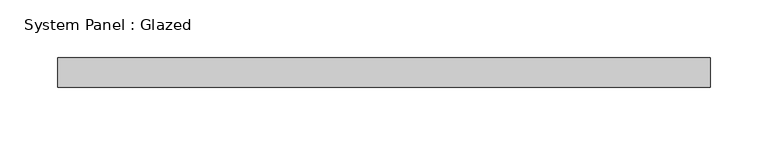
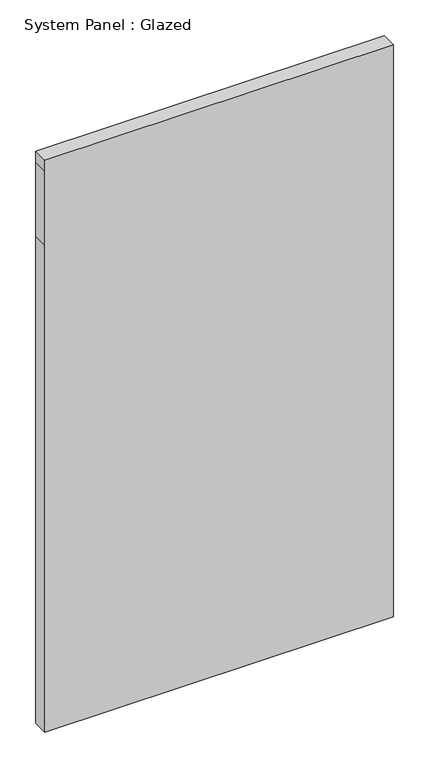
"""IFC4 building model written with IfcOpenShell, lengths in millimetres: plate geometry, System Panel : Glazed."""

from ifc_helpers import new_model, si_unit, frame, origin, place, context, project, spatial, polyline, outline, extrude, source, transform, mapped, element, save


def system_panel_glazed_82992491(model_context):
    return source(origin(), model_context, "Body", "SweptSolid", [
        extrude(outline(polyline([(0.0, -282.575), (0.0, 282.575), (833.9039078, 282.575), (960.9039078, 282.575), (979.9539078, 282.575), (979.9539078, -282.575), (960.9039078, -282.575), (833.9039078, -282.575), (0.0, -282.575)])), frame((0.0, 19.05, 0.0), z_axis=(0.0, 1.0, 0.0), x_axis=(0.0, 0.0, 1.0)), (0.0, 0.0, 1.0), 25.4),
    ])


if __name__ == "__main__":
    model = new_model("IFC4")
    model_context = context("Model", 3, world=origin())
    ifc_project = project(units=[si_unit("LENGTHUNIT", "METRE", prefix="MILLI")], contexts=[model_context])
    site = spatial("IfcSite", under=ifc_project)
    building = spatial("IfcBuilding", under=site)
    placement = place(None, origin())
    system_panel_glazed_shape = system_panel_glazed_82992491(model_context)
    element("IfcPlate", 1, ObjectType="System Panel : Glazed", at=placement, inside=building, context=model_context, shape_type="MappedRepresentation", body=[
        mapped(system_panel_glazed_shape, transform((0.0, 0.0, 0.0), x_axis=(1.0, 0.0, 0.0), y_axis=(0.0, 1.0, 0.0), z_axis=(0.0, 0.0, 1.0))),
    ])
    save(model, "model.ifc")

# Revit data of these elements
# Type "System Panel : Glazed"
#   Construction Type Id = "GSP4R"
#   Analytic Construction = "1/8 in Pilkington single glazing"
#   Visual Light Transmittance = 0.9
#   Solar Heat Gain Coefficient = 0.86
#   Heat Transfer Coefficient (U) = 1.18115 BTU/(h·ft²·°F)
#   Define Thermal Properties by = 1
# Element 1 (IfcPlate, "System Panel : Glazed")
#   Materials on its faces: "Glass"
# Materials
#   "Glass": class "Glass", colour RGB 0 128 192, transparency 0.75, Description = "Soda Lime Glass", Cost = 0
